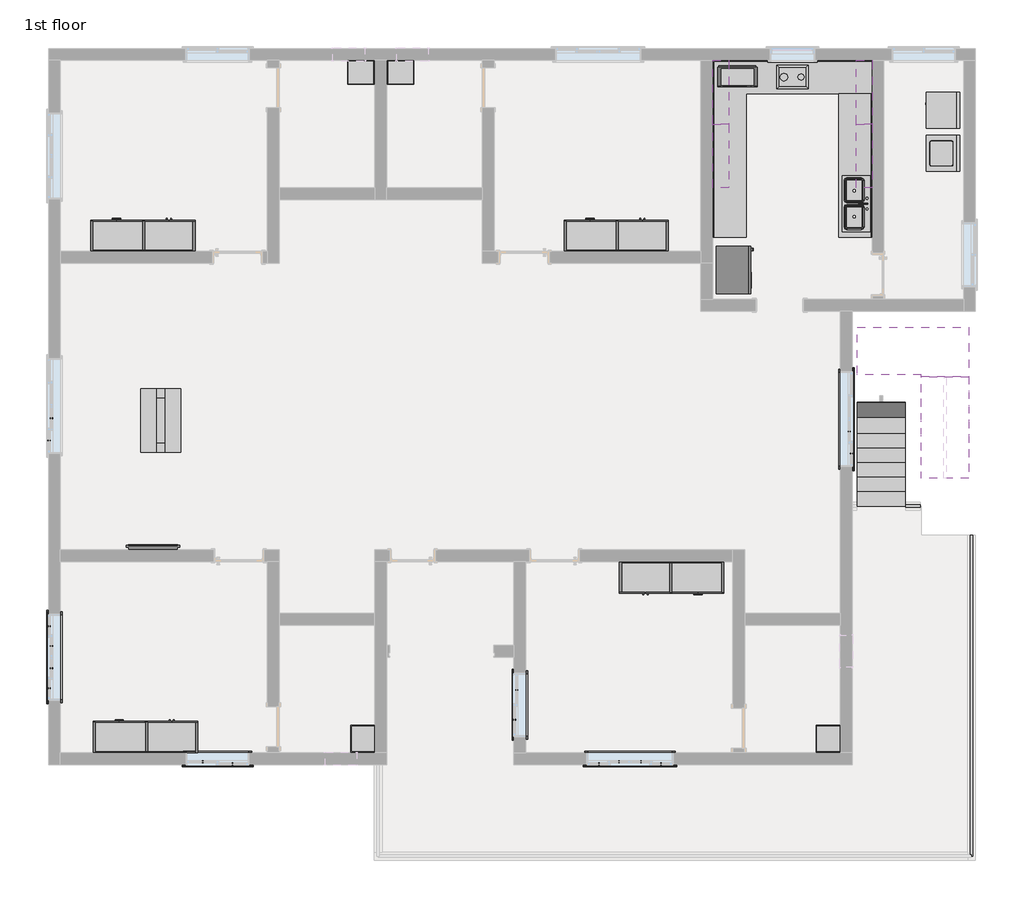
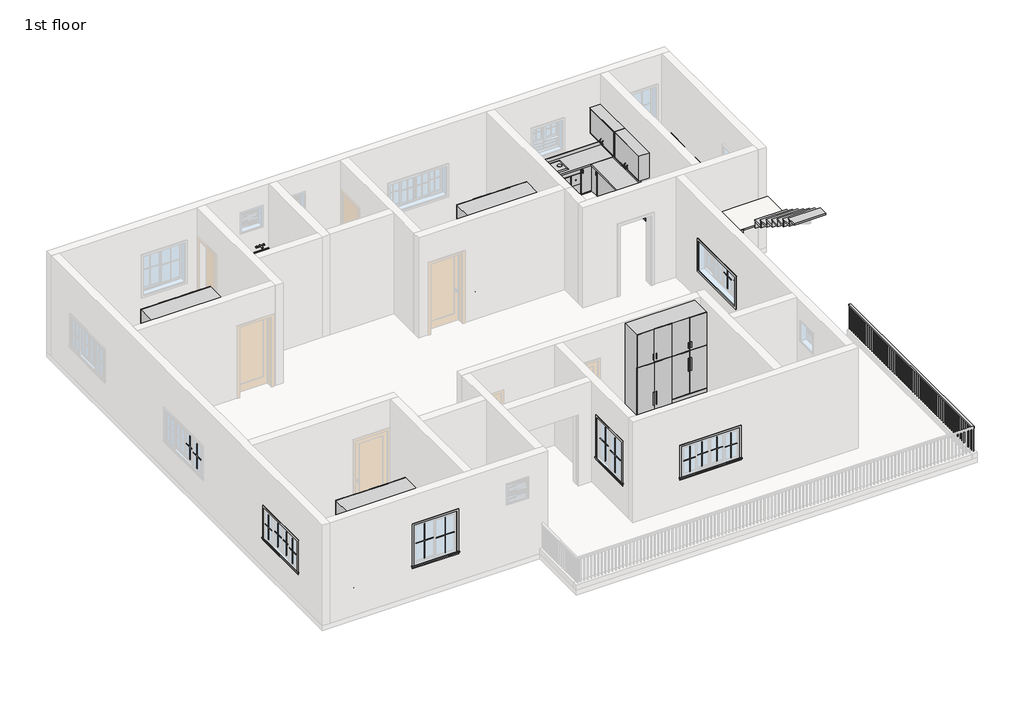
# One storey, part 3 of 4: 30 proxies, 19 furniture elements, 5 flow terminals, 2 railings, 2 stair flights, 1 slab.
"""IFC4 building model written with IfcOpenShell, lengths in millimetres."""

from ifc_helpers import new_model, si_unit, frame, origin, place, context, project, spatial, polyline, outline, extrude, transform, mapped, element, save
from components import proxy_3c1fa1d0, proxy_97c73763, proxy_e661f726, muntin_pattern_2x2_muntin_pattern_2x2_6186d23a, muntin_pattern_2x2_muntin_pattern_2x2_31a16349, muntin_pattern_2x2_muntin_pattern_2x2_cf37b409, trim_window_exterior_flat_with_sill_c3f87112, trim_window_exterior_flat_with_sill_3c945769, trim_window_exterior_flat_with_sill_7cfdd449, trim_window_interior_flat_picture_frame_1c33fa8a, trim_window_interior_flat_picture_frame_0edfbaa2, trim_window_interior_flat_picture_frame_f1e0b15b, proxy_e75280ca, flow_terminal_cce4e9d2, flow_terminal_a53be723, furniture_65fa61b5, furniture_1wardrobe_6271_1wardrobe_6271_4dd35231, furniture_3428e43d, furniture_97fe820d, furniture_803bf5e8, furniture_2797bbf7, furniture_b6aab1a0, furniture_ea954fa4, white_modern_coffee_table_17067_white_modern_coffee_table_d4aed9ff, non_monolithic_landing_cef278ae, stair_flight_508a9823, stair_flight_95b2deb1

model = new_model("IFC4")

# Units and contexts
model_context = context("Model", 3, world=origin())
ifc_project = project(units=[si_unit("LENGTHUNIT", "METRE", prefix="MILLI")], contexts=[model_context])

# Site, building, storey
site = spatial("IfcSite", under=ifc_project)
building = spatial("IfcBuilding", under=site)
storey = spatial("IfcBuildingStorey", under=building, Name="1st floor", Elevation=3810.0)

# Proxies
placement = place(None, origin())
proxy_shape = proxy_3c1fa1d0(model_context)
element("IfcBuildingElementProxy", 1, Name="Cook Top-2 Unit : 12\" x 18\" 2", ObjectType="Cook Top-2 Unit : 12\" x 18\" 2", at=placement, inside=storey, context=model_context, shape_type="MappedRepresentation", body=[
    mapped(proxy_shape, transform((6250.0508793, 6451.6660813, 3810.0), x_axis=(0.0, 1.0, 0.0), y_axis=(-1.0, 0.0, 0.0), z_axis=(0.0, 0.0, 1.0))),
])
proxy_2_shape = proxy_97c73763(model_context)
element("IfcBuildingElementProxy", 2, Name="Dryer : 27\" x 25\" x 35\"", ObjectType="Dryer : 27\" x 25\" x 35\"", at=placement, inside=storey, context=model_context, shape_type="MappedRepresentation", body=[
    mapped(proxy_2_shape, transform((8788.3284624, 6271.8535376, 3810.0), x_axis=(0.0, -1.0, 0.0), y_axis=(1.0, 0.0, 0.0), z_axis=(0.0, 0.0, 1.0))),
])
proxy_3_shape = proxy_e661f726(model_context)
element("IfcBuildingElementProxy", 3, Name="Microwave : 30\" x 16\" x 18\"", ObjectType="Microwave : 30\" x 16\" x 18\"", at=placement, inside=storey, context=model_context, shape_type="MappedRepresentation", body=[
    mapped(proxy_3_shape, transform((4665.4332064, 6893.6465872, 3810.0), x_axis=(1.0, 0.0, 0.0), y_axis=(0.0, 1.0, 0.0), z_axis=(0.0, 0.0, 1.0))),
])
muntin_pattern_2x2_muntin_pattern_2x2_shape = muntin_pattern_2x2_muntin_pattern_2x2_6186d23a(model_context)
element("IfcBuildingElementProxy", 4, Name="Muntin Pattern_2x2 : Muntin Pattern_2x2", ObjectType="Muntin Pattern_2x2 : Muntin Pattern_2x2", at=placement, inside=storey, context=model_context, shape_type="MappedRepresentation", body=[
    mapped(muntin_pattern_2x2_muntin_pattern_2x2_shape, transform((3702.0510838, -6632.5089187, 4806.95), x_axis=(-1.0, 0.0, 0.0), y_axis=(0.0, -1.0, 0.0), z_axis=(0.0, 0.0, 1.0))),
])
element("IfcBuildingElementProxy", 5, Name="Muntin Pattern_2x2 : Muntin Pattern_2x2", ObjectType="Muntin Pattern_2x2 : Muntin Pattern_2x2", at=placement, inside=storey, context=model_context, shape_type="MappedRepresentation", body=[
    mapped(muntin_pattern_2x2_muntin_pattern_2x2_shape, transform((3321.0510838, -6588.0589187, 4806.95), x_axis=(-1.0, 0.0, 0.0), y_axis=(0.0, -1.0, 0.0), z_axis=(0.0, 0.0, 1.0))),
])
element("IfcBuildingElementProxy", 6, Name="Muntin Pattern_2x2 : Muntin Pattern_2x2", ObjectType="Muntin Pattern_2x2 : Muntin Pattern_2x2", at=placement, inside=storey, context=model_context, shape_type="MappedRepresentation", body=[
    mapped(muntin_pattern_2x2_muntin_pattern_2x2_shape, transform((2895.6010838, -6588.0589187, 4806.95), x_axis=(-1.0, 0.0, 0.0), y_axis=(0.0, -1.0, 0.0), z_axis=(0.0, 0.0, 1.0))),
])
element("IfcBuildingElementProxy", 7, Name="Muntin Pattern_2x2 : Muntin Pattern_2x2", ObjectType="Muntin Pattern_2x2 : Muntin Pattern_2x2", at=placement, inside=storey, context=model_context, shape_type="MappedRepresentation", body=[
    mapped(muntin_pattern_2x2_muntin_pattern_2x2_shape, transform((2514.6010838, -6632.5089187, 4806.95), x_axis=(-1.0, 0.0, 0.0), y_axis=(0.0, -1.0, 0.0), z_axis=(0.0, 0.0, 1.0))),
])
element("IfcBuildingElementProxy", 8, Name="Muntin Pattern_2x2 : Muntin Pattern_2x2", ObjectType="Muntin Pattern_2x2 : Muntin Pattern_2x2", at=placement, inside=storey, context=model_context, shape_type="MappedRepresentation", body=[
    mapped(muntin_pattern_2x2_muntin_pattern_2x2_shape, transform((-8020.0489162, -5178.3589187, 4806.95), x_axis=(0.0, 1.0, 0.0), y_axis=(-1.0, 0.0, 0.0), z_axis=(0.0, 0.0, 1.0))),
])
element("IfcBuildingElementProxy", 9, Name="Muntin Pattern_2x2 : Muntin Pattern_2x2", ObjectType="Muntin Pattern_2x2 : Muntin Pattern_2x2", at=placement, inside=storey, context=model_context, shape_type="MappedRepresentation", body=[
    mapped(muntin_pattern_2x2_muntin_pattern_2x2_shape, transform((-7975.5989162, -4797.3589187, 4806.95), x_axis=(0.0, 1.0, 0.0), y_axis=(-1.0, 0.0, 0.0), z_axis=(0.0, 0.0, 1.0))),
])
element("IfcBuildingElementProxy", 10, Name="Muntin Pattern_2x2 : Muntin Pattern_2x2", ObjectType="Muntin Pattern_2x2 : Muntin Pattern_2x2", at=placement, inside=storey, context=model_context, shape_type="MappedRepresentation", body=[
    mapped(muntin_pattern_2x2_muntin_pattern_2x2_shape, transform((-7975.5989162, -4371.9089187, 4806.95), x_axis=(0.0, 1.0, 0.0), y_axis=(-1.0, 0.0, 0.0), z_axis=(0.0, 0.0, 1.0))),
])
element("IfcBuildingElementProxy", 11, Name="Muntin Pattern_2x2 : Muntin Pattern_2x2", ObjectType="Muntin Pattern_2x2 : Muntin Pattern_2x2", at=placement, inside=storey, context=model_context, shape_type="MappedRepresentation", body=[
    mapped(muntin_pattern_2x2_muntin_pattern_2x2_shape, transform((-8020.0489162, -3990.9089187, 4806.95), x_axis=(0.0, 1.0, 0.0), y_axis=(-1.0, 0.0, 0.0), z_axis=(0.0, 0.0, 1.0))),
])
muntin_pattern_2x2_muntin_pattern_2x2_2_shape = muntin_pattern_2x2_muntin_pattern_2x2_31a16349(model_context)
element("IfcBuildingElementProxy", 12, Name="Muntin Pattern_2x2 : Muntin Pattern_2x2", ObjectType="Muntin Pattern_2x2 : Muntin Pattern_2x2", at=placement, inside=storey, context=model_context, shape_type="MappedRepresentation", body=[
    mapped(muntin_pattern_2x2_muntin_pattern_2x2_2_shape, transform((-8020.0489162, -431.7339187, 4806.95), x_axis=(0.0, 1.0, 0.0), y_axis=(-1.0, 0.0, 0.0), z_axis=(0.0, 0.0, 1.0))),
])
element("IfcBuildingElementProxy", 13, Name="Muntin Pattern_2x2 : Muntin Pattern_2x2", ObjectType="Muntin Pattern_2x2 : Muntin Pattern_2x2", at=placement, inside=storey, context=model_context, shape_type="MappedRepresentation", body=[
    mapped(muntin_pattern_2x2_muntin_pattern_2x2_2_shape, transform((-7975.5989162, -6.2839187, 4806.95), x_axis=(0.0, 1.0, 0.0), y_axis=(-1.0, 0.0, 0.0), z_axis=(0.0, 0.0, 1.0))),
])
element("IfcBuildingElementProxy", 14, Name="Muntin Pattern_2x2 : Muntin Pattern_2x2", ObjectType="Muntin Pattern_2x2 : Muntin Pattern_2x2", at=placement, inside=storey, context=model_context, shape_type="MappedRepresentation", body=[
    mapped(muntin_pattern_2x2_muntin_pattern_2x2_2_shape, transform((7308.8510838, -260.2839187, 4806.95), x_axis=(0.0, -1.0, 0.0), y_axis=(1.0, 0.0, 0.0), z_axis=(0.0, 0.0, 1.0))),
])
element("IfcBuildingElementProxy", 15, Name="Muntin Pattern_2x2 : Muntin Pattern_2x2", ObjectType="Muntin Pattern_2x2 : Muntin Pattern_2x2", at=placement, inside=storey, context=model_context, shape_type="MappedRepresentation", body=[
    mapped(muntin_pattern_2x2_muntin_pattern_2x2_2_shape, transform((7353.3010838, -685.7339187, 4806.95), x_axis=(0.0, -1.0, 0.0), y_axis=(1.0, 0.0, 0.0), z_axis=(0.0, 0.0, 1.0))),
])
muntin_pattern_2x2_muntin_pattern_2x2_3_shape = muntin_pattern_2x2_muntin_pattern_2x2_cf37b409(model_context)
element("IfcBuildingElementProxy", 16, Name="Muntin Pattern_2x2 : Muntin Pattern_2x2", ObjectType="Muntin Pattern_2x2 : Muntin Pattern_2x2", at=placement, inside=storey, context=model_context, shape_type="MappedRepresentation", body=[
    mapped(muntin_pattern_2x2_muntin_pattern_2x2_3_shape, transform((939.8010838, -5214.8714187, 4806.95), x_axis=(0.0, 1.0, 0.0), y_axis=(-1.0, 0.0, 0.0), z_axis=(0.0, 0.0, 1.0))),
])
element("IfcBuildingElementProxy", 17, Name="Muntin Pattern_2x2 : Muntin Pattern_2x2", ObjectType="Muntin Pattern_2x2 : Muntin Pattern_2x2", at=placement, inside=storey, context=model_context, shape_type="MappedRepresentation", body=[
    mapped(muntin_pattern_2x2_muntin_pattern_2x2_3_shape, transform((895.3510838, -5783.1964187, 4806.95), x_axis=(0.0, 1.0, 0.0), y_axis=(-1.0, 0.0, 0.0), z_axis=(0.0, 0.0, 1.0))),
])
element("IfcBuildingElementProxy", 18, Name="Muntin Pattern_2x2 : Muntin Pattern_2x2", ObjectType="Muntin Pattern_2x2 : Muntin Pattern_2x2", at=placement, inside=storey, context=model_context, shape_type="MappedRepresentation", body=[
    mapped(muntin_pattern_2x2_muntin_pattern_2x2_3_shape, transform((-5075.2364162, -6588.0589187, 4806.95), x_axis=(-1.0, 0.0, 0.0), y_axis=(0.0, -1.0, 0.0), z_axis=(0.0, 0.0, 1.0))),
])
element("IfcBuildingElementProxy", 19, Name="Muntin Pattern_2x2 : Muntin Pattern_2x2", ObjectType="Muntin Pattern_2x2 : Muntin Pattern_2x2", at=placement, inside=storey, context=model_context, shape_type="MappedRepresentation", body=[
    mapped(muntin_pattern_2x2_muntin_pattern_2x2_3_shape, transform((-4506.9114162, -6632.5089187, 4806.95), x_axis=(-1.0, 0.0, 0.0), y_axis=(0.0, -1.0, 0.0), z_axis=(0.0, 0.0, 1.0))),
])
trim_window_exterior_flat_with_sill_shape = trim_window_exterior_flat_with_sill_c3f87112(model_context)
element("IfcBuildingElementProxy", 20, Name="Trim-Window-Exterior-Flat : with Sill", ObjectType="Trim-Window-Exterior-Flat : with Sill", at=placement, inside=storey, context=model_context, shape_type="MappedRepresentation", body=[
    mapped(trim_window_exterior_flat_with_sill_shape, transform((3108.3260838, -6642.0339187, 5638.8), x_axis=(1.0, 0.0, 0.0), y_axis=(0.0, 0.0, 1.0), z_axis=(0.0, -1.0, 0.0))),
])
element("IfcBuildingElementProxy", 21, Name="Trim-Window-Exterior-Flat : with Sill", ObjectType="Trim-Window-Exterior-Flat : with Sill", at=placement, inside=storey, context=model_context, shape_type="MappedRepresentation", body=[
    mapped(trim_window_exterior_flat_with_sill_shape, transform((-8029.5739162, -4584.6339187, 5638.8), x_axis=(0.0, -1.0, 0.0), y_axis=(0.0, 0.0, 1.0), z_axis=(-1.0, 0.0, 0.0))),
])
trim_window_exterior_flat_with_sill_2_shape = trim_window_exterior_flat_with_sill_3c945769(model_context)
element("IfcBuildingElementProxy", 22, Name="Trim-Window-Exterior-Flat : with Sill", ObjectType="Trim-Window-Exterior-Flat : with Sill", at=placement, inside=storey, context=model_context, shape_type="MappedRepresentation", body=[
    mapped(trim_window_exterior_flat_with_sill_2_shape, transform((7362.8260838, -25.3339187, 5638.8), x_axis=(0.0, 1.0, 0.0), y_axis=(0.0, 0.0, 1.0), z_axis=(1.0, 0.0, 0.0))),
])
trim_window_exterior_flat_with_sill_3_shape = trim_window_exterior_flat_with_sill_7cfdd449(model_context)
element("IfcBuildingElementProxy", 23, Name="Trim-Window-Exterior-Flat : with Sill", ObjectType="Trim-Window-Exterior-Flat : with Sill", at=placement, inside=storey, context=model_context, shape_type="MappedRepresentation", body=[
    mapped(trim_window_exterior_flat_with_sill_3_shape, transform((885.8260838, -5499.0339187, 5943.6), x_axis=(0.0, -1.0, 0.0), y_axis=(0.0, 0.0, 1.0), z_axis=(-1.0, 0.0, 0.0))),
])
element("IfcBuildingElementProxy", 24, Name="Trim-Window-Exterior-Flat : with Sill", ObjectType="Trim-Window-Exterior-Flat : with Sill", at=placement, inside=storey, context=model_context, shape_type="MappedRepresentation", body=[
    mapped(trim_window_exterior_flat_with_sill_3_shape, transform((-4791.0739162, -6642.0339187, 5943.6), x_axis=(1.0, 0.0, 0.0), y_axis=(0.0, 0.0, 1.0), z_axis=(0.0, -1.0, 0.0))),
])
trim_window_interior_flat_picture_frame_shape = trim_window_interior_flat_picture_frame_1c33fa8a(model_context)
element("IfcBuildingElementProxy", 25, Name="Trim-Window-Interior-Flat : Picture Frame", ObjectType="Trim-Window-Interior-Flat : Picture Frame", at=placement, inside=storey, context=model_context, shape_type="MappedRepresentation", body=[
    mapped(trim_window_interior_flat_picture_frame_shape, transform((3108.3260838, -6413.4339187, 5638.8), x_axis=(-1.0, 0.0, 0.0), y_axis=(0.0, 0.0, 1.0), z_axis=(0.0, 1.0, 0.0))),
])
element("IfcBuildingElementProxy", 26, Name="Trim-Window-Interior-Flat : Picture Frame", ObjectType="Trim-Window-Interior-Flat : Picture Frame", at=placement, inside=storey, context=model_context, shape_type="MappedRepresentation", body=[
    mapped(trim_window_interior_flat_picture_frame_shape, transform((-7800.9739162, -4584.6339187, 5638.8), x_axis=(0.0, 1.0, 0.0), y_axis=(0.0, 0.0, 1.0), z_axis=(1.0, 0.0, 0.0))),
])
trim_window_interior_flat_picture_frame_2_shape = trim_window_interior_flat_picture_frame_0edfbaa2(model_context)
element("IfcBuildingElementProxy", 27, Name="Trim-Window-Interior-Flat : Picture Frame", ObjectType="Trim-Window-Interior-Flat : Picture Frame", at=placement, inside=storey, context=model_context, shape_type="MappedRepresentation", body=[
    mapped(trim_window_interior_flat_picture_frame_2_shape, transform((7134.2260838, -25.3339187, 5638.8), x_axis=(0.0, -1.0, 0.0), y_axis=(0.0, 0.0, 1.0), z_axis=(-1.0, 0.0, 0.0))),
])
trim_window_interior_flat_picture_frame_3_shape = trim_window_interior_flat_picture_frame_f1e0b15b(model_context)
element("IfcBuildingElementProxy", 28, Name="Trim-Window-Interior-Flat : Picture Frame", ObjectType="Trim-Window-Interior-Flat : Picture Frame", at=placement, inside=storey, context=model_context, shape_type="MappedRepresentation", body=[
    mapped(trim_window_interior_flat_picture_frame_3_shape, transform((1114.4260838, -5499.0339187, 5943.6), x_axis=(0.0, 1.0, 0.0), y_axis=(0.0, 0.0, 1.0), z_axis=(1.0, 0.0, 0.0))),
])
element("IfcBuildingElementProxy", 29, Name="Trim-Window-Interior-Flat : Picture Frame", ObjectType="Trim-Window-Interior-Flat : Picture Frame", at=placement, inside=storey, context=model_context, shape_type="MappedRepresentation", body=[
    mapped(trim_window_interior_flat_picture_frame_3_shape, transform((-4791.0739162, -6413.4339187, 5943.6), x_axis=(-1.0, 0.0, 0.0), y_axis=(0.0, 0.0, 1.0), z_axis=(0.0, 1.0, 0.0))),
])
proxy_4_shape = proxy_e75280ca(model_context)
element("IfcBuildingElementProxy", 30, Name="Washer : 27\" x 25\" x 35\"", ObjectType="Washer : 27\" x 25\" x 35\"", at=placement, inside=storey, context=model_context, shape_type="MappedRepresentation", body=[
    mapped(proxy_4_shape, transform((8824.6435523, 5486.2156461, 3810.0), x_axis=(0.0, -1.0, 0.0), y_axis=(1.0, 0.0, 0.0), z_axis=(0.0, 0.0, 1.0))),
])

# Flow terminals
flow_terminal_shape = flow_terminal_cce4e9d2(model_context)
element("IfcFlowTerminal", 31, ObjectType="Sink - Work : 20\"x18\"", at=placement, inside=storey, context=model_context, shape_type="MappedRepresentation", body=[
    mapped(flow_terminal_shape, transform((-1285.8739162, 6845.3660813, 4724.4), x_axis=(1.0, 0.0, 0.0), y_axis=(0.0, 1.0, 0.0), z_axis=(0.0, 0.0, 1.0))),
])
element("IfcFlowTerminal", 32, ObjectType="Sink - Work : 20\"x18\"", at=placement, inside=storey, context=model_context, shape_type="MappedRepresentation", body=[
    mapped(flow_terminal_shape, transform((-2047.8739162, 6845.3660813, 4724.4), x_axis=(1.0, 0.0, 0.0), y_axis=(0.0, 1.0, 0.0), z_axis=(0.0, 0.0, 1.0))),
])
element("IfcFlowTerminal", 33, ObjectType="Sink - Work : 20\"x18\"", at=placement, inside=storey, context=model_context, shape_type="MappedRepresentation", body=[
    mapped(flow_terminal_shape, transform((-1781.1739162, -6146.7339187, 4724.4), x_axis=(0.0, -1.0, 0.0), y_axis=(1.0, 0.0, 0.0), z_axis=(0.0, 0.0, 1.0))),
])
element("IfcFlowTerminal", 34, ObjectType="Sink - Work : 20\"x18\"", at=placement, inside=storey, context=model_context, shape_type="MappedRepresentation", body=[
    mapped(flow_terminal_shape, transform((7134.2260838, -6146.7339187, 4724.4), x_axis=(0.0, -1.0, 0.0), y_axis=(1.0, 0.0, 0.0), z_axis=(0.0, 0.0, 1.0))),
])
flow_terminal_2_shape = flow_terminal_a53be723(model_context)
element("IfcFlowTerminal", 35, ObjectType="Sink Kitchen-Double : 42\" x 21\"", at=placement, inside=storey, context=model_context, shape_type="MappedRepresentation", body=[
    mapped(flow_terminal_2_shape, transform((7436.6806826, 4117.8553219, 3810.0), x_axis=(0.0, -1.0, 0.0), y_axis=(1.0, 0.0, 0.0), z_axis=(0.0, 0.0, 1.0))),
])

# Furniture
furniture_shape = furniture_65fa61b5(model_context)
element("IfcFurniture", 36, at=placement, inside=storey, context=model_context, shape_type="MappedRepresentation", body=[
    mapped(furniture_shape, transform((4759.3260838, 3441.7660813, 3810.0), x_axis=(0.0, 1.0, 0.0), y_axis=(-1.0, 0.0, 0.0), z_axis=(0.0, 0.0, 1.0))),
])
furniture_1wardrobe_6271_1wardrobe_6271_shape = furniture_1wardrobe_6271_1wardrobe_6271_4dd35231(model_context)
element("IfcFurniture", 37, ObjectType="1Wardrobe_6271 : 1Wardrobe_6271", at=placement, inside=storey, context=model_context, shape_type="MappedRepresentation", body=[
    mapped(furniture_1wardrobe_6271_1wardrobe_6271_shape, transform((-5222.8739162, 3187.7660813, 3810.0), x_axis=(-1.0, 0.0, 0.0), y_axis=(0.0, -1.0, 0.0), z_axis=(0.0, 0.0, 1.0))),
])
element("IfcFurniture", 38, ObjectType="1Wardrobe_6271 : 1Wardrobe_6271", at=placement, inside=storey, context=model_context, shape_type="MappedRepresentation", body=[
    mapped(furniture_1wardrobe_6271_1wardrobe_6271_shape, transform((3844.9260838, 3187.7660813, 3810.0), x_axis=(-1.0, 0.0, 0.0), y_axis=(0.0, -1.0, 0.0), z_axis=(0.0, 0.0, 1.0))),
])
element("IfcFurniture", 39, ObjectType="1Wardrobe_6271 : 1Wardrobe_6271", at=placement, inside=storey, context=model_context, shape_type="MappedRepresentation", body=[
    mapped(furniture_1wardrobe_6271_1wardrobe_6271_shape, transform((2905.1260838, -2755.8339187, 3810.0), x_axis=(1.0, 0.0, 0.0), y_axis=(0.0, 1.0, 0.0), z_axis=(0.0, 0.0, 1.0))),
])
element("IfcFurniture", 40, ObjectType="1Wardrobe_6271 : 1Wardrobe_6271", at=placement, inside=storey, context=model_context, shape_type="MappedRepresentation", body=[
    mapped(furniture_1wardrobe_6271_1wardrobe_6271_shape, transform((-5172.0739162, -6413.4339187, 3810.0), x_axis=(-1.0, 0.0, 0.0), y_axis=(0.0, -1.0, 0.0), z_axis=(0.0, 0.0, 1.0))),
])
furniture_2_shape = furniture_3428e43d(model_context)
element("IfcFurniture", 41, ObjectType="48\" 2", at=placement, inside=storey, context=model_context, shape_type="MappedRepresentation", body=[
    mapped(furniture_2_shape, transform((6128.9811238, 6845.3660813, 3810.0), x_axis=(1.0, 0.0, 0.0), y_axis=(0.0, 1.0, 0.0), z_axis=(0.0, 0.0, 1.0))),
])
element("IfcFurniture", 42, ObjectType="48\" 2", at=placement, inside=storey, context=model_context, shape_type="MappedRepresentation", body=[
    mapped(furniture_2_shape, transform((7134.2260838, 5230.5211213, 3810.0), x_axis=(0.0, 1.0, 0.0), y_axis=(-1.0, 0.0, 0.0), z_axis=(0.0, 0.0, 1.0))),
])
element("IfcFurniture", 43, ObjectType="48\" 2", at=placement, inside=storey, context=model_context, shape_type="MappedRepresentation", body=[
    mapped(furniture_2_shape, transform((4695.8260838, 5230.5211213, 3810.0), x_axis=(0.0, 1.0, 0.0), y_axis=(-1.0, 0.0, 0.0), z_axis=(0.0, 0.0, 1.0))),
])
element("IfcFurniture", 44, ObjectType="48\" 2", at=placement, inside=storey, context=model_context, shape_type="MappedRepresentation", body=[
    mapped(furniture_2_shape, transform((4695.8260838, 4011.3211213, 3810.0), x_axis=(0.0, 1.0, 0.0), y_axis=(-1.0, 0.0, 0.0), z_axis=(0.0, 0.0, 1.0))),
])
furniture_3_shape = furniture_97fe820d(model_context)
element("IfcFurniture", 45, ObjectType="Base Cabinet-Corner Unit-Square : 36\"", at=placement, inside=storey, context=model_context, shape_type="MappedRepresentation", body=[
    mapped(furniture_3_shape, transform((7217.0883788, 6845.3660813, 3810.0), x_axis=(1.0, 0.0, 0.0), y_axis=(0.0, 1.0, 0.0), z_axis=(0.0, 0.0, 1.0))),
])
element("IfcFurniture", 46, ObjectType="Base Cabinet-Corner Unit-Square : 36\"", at=placement, inside=storey, context=model_context, shape_type="MappedRepresentation", body=[
    mapped(furniture_3_shape, transform((4695.8260838, 6318.6283764, 3810.0), x_axis=(0.0, 1.0, 0.0), y_axis=(-1.0, 0.0, 0.0), z_axis=(0.0, 0.0, 1.0))),
])
furniture_4_shape = furniture_803bf5e8(model_context)
element("IfcFurniture", 47, ObjectType="Counter Top w Sink : 24\" Depth", at=placement, inside=storey, context=model_context, shape_type="MappedRepresentation", body=[
    mapped(furniture_4_shape, transform((7743.8260838, 5009.9037862, 3810.0), x_axis=(0.0, -1.0, 0.0), y_axis=(1.0, 0.0, 0.0), z_axis=(0.0, 0.0, 1.0))),
])
furniture_5_shape = furniture_2797bbf7(model_context)
element("IfcFurniture", 48, ObjectType="Counter Top-L Shaped : 24\" Depth", at=placement, inside=storey, context=model_context, shape_type="MappedRepresentation", body=[
    mapped(furniture_5_shape, transform((5896.2883788, 6845.3660813, 3810.0), x_axis=(1.0, 0.0, 0.0), y_axis=(0.0, 1.0, 0.0), z_axis=(0.0, 0.0, 1.0))),
])
furniture_6_shape = furniture_b6aab1a0(model_context)
element("IfcFurniture", 49, ObjectType="Television-Plasma : 42\"", at=placement, inside=storey, context=model_context, shape_type="MappedRepresentation", body=[
    mapped(furniture_6_shape, transform((-5972.1739162, -2527.2339187, 4876.8), x_axis=(-1.0, 0.0, 0.0), y_axis=(0.0, -1.0, 0.0), z_axis=(0.0, 0.0, 1.0))),
])
furniture_7_shape = furniture_ea954fa4(model_context)
element("IfcFurniture", 50, ObjectType="Upper Cabinet-Pass-Thru : 48\" x 30\" x 12\"", at=placement, inside=storey, context=model_context, shape_type="MappedRepresentation", body=[
    mapped(furniture_7_shape, transform((4695.8260838, 6217.0283764, 3810.0), x_axis=(0.0, 1.0, 0.0), y_axis=(-1.0, 0.0, 0.0), z_axis=(0.0, 0.0, 1.0))),
])
element("IfcFurniture", 51, ObjectType="Upper Cabinet-Pass-Thru : 48\" x 30\" x 12\"", at=placement, inside=storey, context=model_context, shape_type="MappedRepresentation", body=[
    mapped(furniture_7_shape, transform((4695.8260838, 4997.8283764, 3810.0), x_axis=(0.0, 1.0, 0.0), y_axis=(-1.0, 0.0, 0.0), z_axis=(0.0, 0.0, 1.0))),
])
element("IfcFurniture", 52, ObjectType="Upper Cabinet-Pass-Thru : 48\" x 30\" x 12\"", at=placement, inside=storey, context=model_context, shape_type="MappedRepresentation", body=[
    mapped(furniture_7_shape, transform((7743.8260838, 6254.5037862, 3810.0), x_axis=(0.0, -1.0, 0.0), y_axis=(1.0, 0.0, 0.0), z_axis=(0.0, 0.0, 1.0))),
])
element("IfcFurniture", 53, ObjectType="Upper Cabinet-Pass-Thru : 48\" x 30\" x 12\"", at=placement, inside=storey, context=model_context, shape_type="MappedRepresentation", body=[
    mapped(furniture_7_shape, transform((7743.8260838, 5035.3037862, 3810.0), x_axis=(0.0, -1.0, 0.0), y_axis=(1.0, 0.0, 0.0), z_axis=(0.0, 0.0, 1.0))),
])
white_modern_coffee_table_17067_white_modern_coffee_table_shape = white_modern_coffee_table_17067_white_modern_coffee_table_d4aed9ff(model_context)
element("IfcFurniture", 54, ObjectType="White_Modern_Coffee_Table_17067 : White_Modern_Coffee_Table_17067", at=placement, inside=storey, context=model_context, shape_type="MappedRepresentation", body=[
    mapped(white_modern_coffee_table_17067_white_modern_coffee_table_shape, transform((-5878.4127262, -50.7339187, 3810.0), x_axis=(0.0, 1.0, 0.0), y_axis=(-1.0, 0.0, 0.0), z_axis=(0.0, 0.0, 1.0))),
])

# Railings
element("IfcRailing", 55, ObjectType="Handrail - Rectangular", at=placement, inside=storey, context=model_context, shape_type="SweptSolid", body=[
    extrude(outline(polyline([(9623.4260838, -2247.8339187), (9674.2260838, -2247.8339187), (9674.2260838, -8394.6339187), (9623.4260838, -8394.6339187), (9623.4260838, -2247.8339187)])), frame((0.0, 0.0, 4673.6), z_axis=(0.0, 0.0, 1.0), x_axis=(1.0, 0.0, 0.0)), (0.0, 0.0, 1.0), 50.8),
    extrude(outline(polyline([(9639.3010838, -8334.3089187), (9658.3510838, -8334.3089187), (9658.3510838, -8353.3589187), (9639.3010838, -8353.3589187), (9639.3010838, -8334.3089187)])), frame((0.0, 0.0, 3810.0), z_axis=(0.0, 0.0, 1.0), x_axis=(1.0, 0.0, 0.0)), (0.0, 0.0, 1.0), 863.6),
    extrude(outline(polyline([(9639.3010838, -8232.7089187), (9658.3510838, -8232.7089187), (9658.3510838, -8251.7589187), (9639.3010838, -8251.7589187), (9639.3010838, -8232.7089187)])), frame((0.0, 0.0, 3810.0), z_axis=(0.0, 0.0, 1.0), x_axis=(1.0, 0.0, 0.0)), (0.0, 0.0, 1.0), 863.6),
    extrude(outline(polyline([(9639.3010838, -8131.1089187), (9658.3510838, -8131.1089187), (9658.3510838, -8150.1589187), (9639.3010838, -8150.1589187), (9639.3010838, -8131.1089187)])), frame((0.0, 0.0, 3810.0), z_axis=(0.0, 0.0, 1.0), x_axis=(1.0, 0.0, 0.0)), (0.0, 0.0, 1.0), 863.6),
    extrude(outline(polyline([(9639.3010838, -8029.5089187), (9658.3510838, -8029.5089187), (9658.3510838, -8048.5589187), (9639.3010838, -8048.5589187), (9639.3010838, -8029.5089187)])), frame((0.0, 0.0, 3810.0), z_axis=(0.0, 0.0, 1.0), x_axis=(1.0, 0.0, 0.0)), (0.0, 0.0, 1.0), 863.6),
    extrude(outline(polyline([(9639.3010838, -7927.9089187), (9658.3510838, -7927.9089187), (9658.3510838, -7946.9589187), (9639.3010838, -7946.9589187), (9639.3010838, -7927.9089187)])), frame((0.0, 0.0, 3810.0), z_axis=(0.0, 0.0, 1.0), x_axis=(1.0, 0.0, 0.0)), (0.0, 0.0, 1.0), 863.6),
    extrude(outline(polyline([(9639.3010838, -7826.3089187), (9658.3510838, -7826.3089187), (9658.3510838, -7845.3589187), (9639.3010838, -7845.3589187), (9639.3010838, -7826.3089187)])), frame((0.0, 0.0, 3810.0), z_axis=(0.0, 0.0, 1.0), x_axis=(1.0, 0.0, 0.0)), (0.0, 0.0, 1.0), 863.6),
    extrude(outline(polyline([(9639.3010838, -7724.7089187), (9658.3510838, -7724.7089187), (9658.3510838, -7743.7589187), (9639.3010838, -7743.7589187), (9639.3010838, -7724.7089187)])), frame((0.0, 0.0, 3810.0), z_axis=(0.0, 0.0, 1.0), x_axis=(1.0, 0.0, 0.0)), (0.0, 0.0, 1.0), 863.6),
    extrude(outline(polyline([(9639.3010838, -7623.1089187), (9658.3510838, -7623.1089187), (9658.3510838, -7642.1589187), (9639.3010838, -7642.1589187), (9639.3010838, -7623.1089187)])), frame((0.0, 0.0, 3810.0), z_axis=(0.0, 0.0, 1.0), x_axis=(1.0, 0.0, 0.0)), (0.0, 0.0, 1.0), 863.6),
    extrude(outline(polyline([(9639.3010838, -7521.5089187), (9658.3510838, -7521.5089187), (9658.3510838, -7540.5589187), (9639.3010838, -7540.5589187), (9639.3010838, -7521.5089187)])), frame((0.0, 0.0, 3810.0), z_axis=(0.0, 0.0, 1.0), x_axis=(1.0, 0.0, 0.0)), (0.0, 0.0, 1.0), 863.6),
    extrude(outline(polyline([(9639.3010838, -7419.9089187), (9658.3510838, -7419.9089187), (9658.3510838, -7438.9589187), (9639.3010838, -7438.9589187), (9639.3010838, -7419.9089187)])), frame((0.0, 0.0, 3810.0), z_axis=(0.0, 0.0, 1.0), x_axis=(1.0, 0.0, 0.0)), (0.0, 0.0, 1.0), 863.6),
    extrude(outline(polyline([(9639.3010838, -7318.3089187), (9658.3510838, -7318.3089187), (9658.3510838, -7337.3589187), (9639.3010838, -7337.3589187), (9639.3010838, -7318.3089187)])), frame((0.0, 0.0, 3810.0), z_axis=(0.0, 0.0, 1.0), x_axis=(1.0, 0.0, 0.0)), (0.0, 0.0, 1.0), 863.6),
    extrude(outline(polyline([(9639.3010838, -7216.7089187), (9658.3510838, -7216.7089187), (9658.3510838, -7235.7589187), (9639.3010838, -7235.7589187), (9639.3010838, -7216.7089187)])), frame((0.0, 0.0, 3810.0), z_axis=(0.0, 0.0, 1.0), x_axis=(1.0, 0.0, 0.0)), (0.0, 0.0, 1.0), 863.6),
    extrude(outline(polyline([(9639.3010838, -7115.1089187), (9658.3510838, -7115.1089187), (9658.3510838, -7134.1589187), (9639.3010838, -7134.1589187), (9639.3010838, -7115.1089187)])), frame((0.0, 0.0, 3810.0), z_axis=(0.0, 0.0, 1.0), x_axis=(1.0, 0.0, 0.0)), (0.0, 0.0, 1.0), 863.6),
    extrude(outline(polyline([(9639.3010838, -7013.5089187), (9658.3510838, -7013.5089187), (9658.3510838, -7032.5589187), (9639.3010838, -7032.5589187), (9639.3010838, -7013.5089187)])), frame((0.0, 0.0, 3810.0), z_axis=(0.0, 0.0, 1.0), x_axis=(1.0, 0.0, 0.0)), (0.0, 0.0, 1.0), 863.6),
    extrude(outline(polyline([(9639.3010838, -6911.9089187), (9658.3510838, -6911.9089187), (9658.3510838, -6930.9589187), (9639.3010838, -6930.9589187), (9639.3010838, -6911.9089187)])), frame((0.0, 0.0, 3810.0), z_axis=(0.0, 0.0, 1.0), x_axis=(1.0, 0.0, 0.0)), (0.0, 0.0, 1.0), 863.6),
    extrude(outline(polyline([(9639.3010838, -6810.3089187), (9658.3510838, -6810.3089187), (9658.3510838, -6829.3589187), (9639.3010838, -6829.3589187), (9639.3010838, -6810.3089187)])), frame((0.0, 0.0, 3810.0), z_axis=(0.0, 0.0, 1.0), x_axis=(1.0, 0.0, 0.0)), (0.0, 0.0, 1.0), 863.6),
    extrude(outline(polyline([(9639.3010838, -6708.7089187), (9658.3510838, -6708.7089187), (9658.3510838, -6727.7589187), (9639.3010838, -6727.7589187), (9639.3010838, -6708.7089187)])), frame((0.0, 0.0, 3810.0), z_axis=(0.0, 0.0, 1.0), x_axis=(1.0, 0.0, 0.0)), (0.0, 0.0, 1.0), 863.6),
    extrude(outline(polyline([(9639.3010838, -6607.1089187), (9658.3510838, -6607.1089187), (9658.3510838, -6626.1589187), (9639.3010838, -6626.1589187), (9639.3010838, -6607.1089187)])), frame((0.0, 0.0, 3810.0), z_axis=(0.0, 0.0, 1.0), x_axis=(1.0, 0.0, 0.0)), (0.0, 0.0, 1.0), 863.6),
    extrude(outline(polyline([(9639.3010838, -6505.5089187), (9658.3510838, -6505.5089187), (9658.3510838, -6524.5589187), (9639.3010838, -6524.5589187), (9639.3010838, -6505.5089187)])), frame((0.0, 0.0, 3810.0), z_axis=(0.0, 0.0, 1.0), x_axis=(1.0, 0.0, 0.0)), (0.0, 0.0, 1.0), 863.6),
    extrude(outline(polyline([(9639.3010838, -6403.9089187), (9658.3510838, -6403.9089187), (9658.3510838, -6422.9589187), (9639.3010838, -6422.9589187), (9639.3010838, -6403.9089187)])), frame((0.0, 0.0, 3810.0), z_axis=(0.0, 0.0, 1.0), x_axis=(1.0, 0.0, 0.0)), (0.0, 0.0, 1.0), 863.6),
    extrude(outline(polyline([(9639.3010838, -6302.3089187), (9658.3510838, -6302.3089187), (9658.3510838, -6321.3589187), (9639.3010838, -6321.3589187), (9639.3010838, -6302.3089187)])), frame((0.0, 0.0, 3810.0), z_axis=(0.0, 0.0, 1.0), x_axis=(1.0, 0.0, 0.0)), (0.0, 0.0, 1.0), 863.6),
    extrude(outline(polyline([(9639.3010838, -6200.7089187), (9658.3510838, -6200.7089187), (9658.3510838, -6219.7589187), (9639.3010838, -6219.7589187), (9639.3010838, -6200.7089187)])), frame((0.0, 0.0, 3810.0), z_axis=(0.0, 0.0, 1.0), x_axis=(1.0, 0.0, 0.0)), (0.0, 0.0, 1.0), 863.6),
    extrude(outline(polyline([(9639.3010838, -6099.1089187), (9658.3510838, -6099.1089187), (9658.3510838, -6118.1589187), (9639.3010838, -6118.1589187), (9639.3010838, -6099.1089187)])), frame((0.0, 0.0, 3810.0), z_axis=(0.0, 0.0, 1.0), x_axis=(1.0, 0.0, 0.0)), (0.0, 0.0, 1.0), 863.6),
    extrude(outline(polyline([(9639.3010838, -5997.5089187), (9658.3510838, -5997.5089187), (9658.3510838, -6016.5589187), (9639.3010838, -6016.5589187), (9639.3010838, -5997.5089187)])), frame((0.0, 0.0, 3810.0), z_axis=(0.0, 0.0, 1.0), x_axis=(1.0, 0.0, 0.0)), (0.0, 0.0, 1.0), 863.6),
    extrude(outline(polyline([(9639.3010838, -5895.9089187), (9658.3510838, -5895.9089187), (9658.3510838, -5914.9589187), (9639.3010838, -5914.9589187), (9639.3010838, -5895.9089187)])), frame((0.0, 0.0, 3810.0), z_axis=(0.0, 0.0, 1.0), x_axis=(1.0, 0.0, 0.0)), (0.0, 0.0, 1.0), 863.6),
    extrude(outline(polyline([(9639.3010838, -5794.3089187), (9658.3510838, -5794.3089187), (9658.3510838, -5813.3589187), (9639.3010838, -5813.3589187), (9639.3010838, -5794.3089187)])), frame((0.0, 0.0, 3810.0), z_axis=(0.0, 0.0, 1.0), x_axis=(1.0, 0.0, 0.0)), (0.0, 0.0, 1.0), 863.6),
    extrude(outline(polyline([(9639.3010838, -5692.7089187), (9658.3510838, -5692.7089187), (9658.3510838, -5711.7589187), (9639.3010838, -5711.7589187), (9639.3010838, -5692.7089187)])), frame((0.0, 0.0, 3810.0), z_axis=(0.0, 0.0, 1.0), x_axis=(1.0, 0.0, 0.0)), (0.0, 0.0, 1.0), 863.6),
    extrude(outline(polyline([(9639.3010838, -5591.1089187), (9658.3510838, -5591.1089187), (9658.3510838, -5610.1589187), (9639.3010838, -5610.1589187), (9639.3010838, -5591.1089187)])), frame((0.0, 0.0, 3810.0), z_axis=(0.0, 0.0, 1.0), x_axis=(1.0, 0.0, 0.0)), (0.0, 0.0, 1.0), 863.6),
    extrude(outline(polyline([(9639.3010838, -5489.5089187), (9658.3510838, -5489.5089187), (9658.3510838, -5508.5589187), (9639.3010838, -5508.5589187), (9639.3010838, -5489.5089187)])), frame((0.0, 0.0, 3810.0), z_axis=(0.0, 0.0, 1.0), x_axis=(1.0, 0.0, 0.0)), (0.0, 0.0, 1.0), 863.6),
    extrude(outline(polyline([(9639.3010838, -5387.9089187), (9658.3510838, -5387.9089187), (9658.3510838, -5406.9589187), (9639.3010838, -5406.9589187), (9639.3010838, -5387.9089187)])), frame((0.0, 0.0, 3810.0), z_axis=(0.0, 0.0, 1.0), x_axis=(1.0, 0.0, 0.0)), (0.0, 0.0, 1.0), 863.6),
    extrude(outline(polyline([(9639.3010838, -5286.3089187), (9658.3510838, -5286.3089187), (9658.3510838, -5305.3589187), (9639.3010838, -5305.3589187), (9639.3010838, -5286.3089187)])), frame((0.0, 0.0, 3810.0), z_axis=(0.0, 0.0, 1.0), x_axis=(1.0, 0.0, 0.0)), (0.0, 0.0, 1.0), 863.6),
    extrude(outline(polyline([(9639.3010838, -5184.7089187), (9658.3510838, -5184.7089187), (9658.3510838, -5203.7589187), (9639.3010838, -5203.7589187), (9639.3010838, -5184.7089187)])), frame((0.0, 0.0, 3810.0), z_axis=(0.0, 0.0, 1.0), x_axis=(1.0, 0.0, 0.0)), (0.0, 0.0, 1.0), 863.6),
    extrude(outline(polyline([(9639.3010838, -5083.1089187), (9658.3510838, -5083.1089187), (9658.3510838, -5102.1589187), (9639.3010838, -5102.1589187), (9639.3010838, -5083.1089187)])), frame((0.0, 0.0, 3810.0), z_axis=(0.0, 0.0, 1.0), x_axis=(1.0, 0.0, 0.0)), (0.0, 0.0, 1.0), 863.6),
    extrude(outline(polyline([(9639.3010838, -4981.5089187), (9658.3510838, -4981.5089187), (9658.3510838, -5000.5589187), (9639.3010838, -5000.5589187), (9639.3010838, -4981.5089187)])), frame((0.0, 0.0, 3810.0), z_axis=(0.0, 0.0, 1.0), x_axis=(1.0, 0.0, 0.0)), (0.0, 0.0, 1.0), 863.6),
    extrude(outline(polyline([(9639.3010838, -4879.9089187), (9658.3510838, -4879.9089187), (9658.3510838, -4898.9589187), (9639.3010838, -4898.9589187), (9639.3010838, -4879.9089187)])), frame((0.0, 0.0, 3810.0), z_axis=(0.0, 0.0, 1.0), x_axis=(1.0, 0.0, 0.0)), (0.0, 0.0, 1.0), 863.6),
    extrude(outline(polyline([(9639.3010838, -4778.3089187), (9658.3510838, -4778.3089187), (9658.3510838, -4797.3589187), (9639.3010838, -4797.3589187), (9639.3010838, -4778.3089187)])), frame((0.0, 0.0, 3810.0), z_axis=(0.0, 0.0, 1.0), x_axis=(1.0, 0.0, 0.0)), (0.0, 0.0, 1.0), 863.6),
    extrude(outline(polyline([(9639.3010838, -4676.7089187), (9658.3510838, -4676.7089187), (9658.3510838, -4695.7589187), (9639.3010838, -4695.7589187), (9639.3010838, -4676.7089187)])), frame((0.0, 0.0, 3810.0), z_axis=(0.0, 0.0, 1.0), x_axis=(1.0, 0.0, 0.0)), (0.0, 0.0, 1.0), 863.6),
    extrude(outline(polyline([(9639.3010838, -4575.1089187), (9658.3510838, -4575.1089187), (9658.3510838, -4594.1589187), (9639.3010838, -4594.1589187), (9639.3010838, -4575.1089187)])), frame((0.0, 0.0, 3810.0), z_axis=(0.0, 0.0, 1.0), x_axis=(1.0, 0.0, 0.0)), (0.0, 0.0, 1.0), 863.6),
    extrude(outline(polyline([(9639.3010838, -4473.5089187), (9658.3510838, -4473.5089187), (9658.3510838, -4492.5589187), (9639.3010838, -4492.5589187), (9639.3010838, -4473.5089187)])), frame((0.0, 0.0, 3810.0), z_axis=(0.0, 0.0, 1.0), x_axis=(1.0, 0.0, 0.0)), (0.0, 0.0, 1.0), 863.6),
    extrude(outline(polyline([(9639.3010838, -4371.9089187), (9658.3510838, -4371.9089187), (9658.3510838, -4390.9589187), (9639.3010838, -4390.9589187), (9639.3010838, -4371.9089187)])), frame((0.0, 0.0, 3810.0), z_axis=(0.0, 0.0, 1.0), x_axis=(1.0, 0.0, 0.0)), (0.0, 0.0, 1.0), 863.6),
    extrude(outline(polyline([(9639.3010838, -4270.3089187), (9658.3510838, -4270.3089187), (9658.3510838, -4289.3589187), (9639.3010838, -4289.3589187), (9639.3010838, -4270.3089187)])), frame((0.0, 0.0, 3810.0), z_axis=(0.0, 0.0, 1.0), x_axis=(1.0, 0.0, 0.0)), (0.0, 0.0, 1.0), 863.6),
    extrude(outline(polyline([(9639.3010838, -4168.7089187), (9658.3510838, -4168.7089187), (9658.3510838, -4187.7589187), (9639.3010838, -4187.7589187), (9639.3010838, -4168.7089187)])), frame((0.0, 0.0, 3810.0), z_axis=(0.0, 0.0, 1.0), x_axis=(1.0, 0.0, 0.0)), (0.0, 0.0, 1.0), 863.6),
    extrude(outline(polyline([(9639.3010838, -4067.1089187), (9658.3510838, -4067.1089187), (9658.3510838, -4086.1589187), (9639.3010838, -4086.1589187), (9639.3010838, -4067.1089187)])), frame((0.0, 0.0, 3810.0), z_axis=(0.0, 0.0, 1.0), x_axis=(1.0, 0.0, 0.0)), (0.0, 0.0, 1.0), 863.6),
    extrude(outline(polyline([(9639.3010838, -3965.5089187), (9658.3510838, -3965.5089187), (9658.3510838, -3984.5589187), (9639.3010838, -3984.5589187), (9639.3010838, -3965.5089187)])), frame((0.0, 0.0, 3810.0), z_axis=(0.0, 0.0, 1.0), x_axis=(1.0, 0.0, 0.0)), (0.0, 0.0, 1.0), 863.6),
    extrude(outline(polyline([(9639.3010838, -3863.9089187), (9658.3510838, -3863.9089187), (9658.3510838, -3882.9589187), (9639.3010838, -3882.9589187), (9639.3010838, -3863.9089187)])), frame((0.0, 0.0, 3810.0), z_axis=(0.0, 0.0, 1.0), x_axis=(1.0, 0.0, 0.0)), (0.0, 0.0, 1.0), 863.6),
    extrude(outline(polyline([(9639.3010838, -3762.3089187), (9658.3510838, -3762.3089187), (9658.3510838, -3781.3589187), (9639.3010838, -3781.3589187), (9639.3010838, -3762.3089187)])), frame((0.0, 0.0, 3810.0), z_axis=(0.0, 0.0, 1.0), x_axis=(1.0, 0.0, 0.0)), (0.0, 0.0, 1.0), 863.6),
    extrude(outline(polyline([(9639.3010838, -3660.7089187), (9658.3510838, -3660.7089187), (9658.3510838, -3679.7589187), (9639.3010838, -3679.7589187), (9639.3010838, -3660.7089187)])), frame((0.0, 0.0, 3810.0), z_axis=(0.0, 0.0, 1.0), x_axis=(1.0, 0.0, 0.0)), (0.0, 0.0, 1.0), 863.6),
    extrude(outline(polyline([(9639.3010838, -3559.1089187), (9658.3510838, -3559.1089187), (9658.3510838, -3578.1589187), (9639.3010838, -3578.1589187), (9639.3010838, -3559.1089187)])), frame((0.0, 0.0, 3810.0), z_axis=(0.0, 0.0, 1.0), x_axis=(1.0, 0.0, 0.0)), (0.0, 0.0, 1.0), 863.6),
    extrude(outline(polyline([(9639.3010838, -3457.5089187), (9658.3510838, -3457.5089187), (9658.3510838, -3476.5589187), (9639.3010838, -3476.5589187), (9639.3010838, -3457.5089187)])), frame((0.0, 0.0, 3810.0), z_axis=(0.0, 0.0, 1.0), x_axis=(1.0, 0.0, 0.0)), (0.0, 0.0, 1.0), 863.6),
    extrude(outline(polyline([(9639.3010838, -3355.9089187), (9658.3510838, -3355.9089187), (9658.3510838, -3374.9589187), (9639.3010838, -3374.9589187), (9639.3010838, -3355.9089187)])), frame((0.0, 0.0, 3810.0), z_axis=(0.0, 0.0, 1.0), x_axis=(1.0, 0.0, 0.0)), (0.0, 0.0, 1.0), 863.6),
    extrude(outline(polyline([(9639.3010838, -3254.3089187), (9658.3510838, -3254.3089187), (9658.3510838, -3273.3589187), (9639.3010838, -3273.3589187), (9639.3010838, -3254.3089187)])), frame((0.0, 0.0, 3810.0), z_axis=(0.0, 0.0, 1.0), x_axis=(1.0, 0.0, 0.0)), (0.0, 0.0, 1.0), 863.6),
    extrude(outline(polyline([(9639.3010838, -3152.7089187), (9658.3510838, -3152.7089187), (9658.3510838, -3171.7589187), (9639.3010838, -3171.7589187), (9639.3010838, -3152.7089187)])), frame((0.0, 0.0, 3810.0), z_axis=(0.0, 0.0, 1.0), x_axis=(1.0, 0.0, 0.0)), (0.0, 0.0, 1.0), 863.6),
    extrude(outline(polyline([(9639.3010838, -3051.1089187), (9658.3510838, -3051.1089187), (9658.3510838, -3070.1589187), (9639.3010838, -3070.1589187), (9639.3010838, -3051.1089187)])), frame((0.0, 0.0, 3810.0), z_axis=(0.0, 0.0, 1.0), x_axis=(1.0, 0.0, 0.0)), (0.0, 0.0, 1.0), 863.6),
    extrude(outline(polyline([(9639.3010838, -2949.5089187), (9658.3510838, -2949.5089187), (9658.3510838, -2968.5589187), (9639.3010838, -2968.5589187), (9639.3010838, -2949.5089187)])), frame((0.0, 0.0, 3810.0), z_axis=(0.0, 0.0, 1.0), x_axis=(1.0, 0.0, 0.0)), (0.0, 0.0, 1.0), 863.6),
    extrude(outline(polyline([(9639.3010838, -2847.9089187), (9658.3510838, -2847.9089187), (9658.3510838, -2866.9589187), (9639.3010838, -2866.9589187), (9639.3010838, -2847.9089187)])), frame((0.0, 0.0, 3810.0), z_axis=(0.0, 0.0, 1.0), x_axis=(1.0, 0.0, 0.0)), (0.0, 0.0, 1.0), 863.6),
    extrude(outline(polyline([(9639.3010838, -2746.3089187), (9658.3510838, -2746.3089187), (9658.3510838, -2765.3589187), (9639.3010838, -2765.3589187), (9639.3010838, -2746.3089187)])), frame((0.0, 0.0, 3810.0), z_axis=(0.0, 0.0, 1.0), x_axis=(1.0, 0.0, 0.0)), (0.0, 0.0, 1.0), 863.6),
    extrude(outline(polyline([(9639.3010838, -2644.7089187), (9658.3510838, -2644.7089187), (9658.3510838, -2663.7589187), (9639.3010838, -2663.7589187), (9639.3010838, -2644.7089187)])), frame((0.0, 0.0, 3810.0), z_axis=(0.0, 0.0, 1.0), x_axis=(1.0, 0.0, 0.0)), (0.0, 0.0, 1.0), 863.6),
    extrude(outline(polyline([(9639.3010838, -2543.1089187), (9658.3510838, -2543.1089187), (9658.3510838, -2562.1589187), (9639.3010838, -2562.1589187), (9639.3010838, -2543.1089187)])), frame((0.0, 0.0, 3810.0), z_axis=(0.0, 0.0, 1.0), x_axis=(1.0, 0.0, 0.0)), (0.0, 0.0, 1.0), 863.6),
    extrude(outline(polyline([(9639.3010838, -2441.5089187), (9658.3510838, -2441.5089187), (9658.3510838, -2460.5589187), (9639.3010838, -2460.5589187), (9639.3010838, -2441.5089187)])), frame((0.0, 0.0, 3810.0), z_axis=(0.0, 0.0, 1.0), x_axis=(1.0, 0.0, 0.0)), (0.0, 0.0, 1.0), 863.6),
    extrude(outline(polyline([(9639.3010838, -2339.9089187), (9658.3510838, -2339.9089187), (9658.3510838, -2358.9589187), (9639.3010838, -2358.9589187), (9639.3010838, -2339.9089187)])), frame((0.0, 0.0, 3810.0), z_axis=(0.0, 0.0, 1.0), x_axis=(1.0, 0.0, 0.0)), (0.0, 0.0, 1.0), 863.6),
    extrude(outline(polyline([(9639.3010838, -8375.5839187), (9658.3510838, -8375.5839187), (9658.3510838, -8394.6339187), (9639.3010838, -8394.6339187), (9639.3010838, -8375.5839187)])), frame((0.0, 0.0, 3810.0), z_axis=(0.0, 0.0, 1.0), x_axis=(1.0, 0.0, 0.0)), (0.0, 0.0, 1.0), 863.6),
    extrude(outline(polyline([(9639.3010838, -2247.8339187), (9658.3510838, -2247.8339187), (9658.3510838, -2266.8839187), (9639.3010838, -2266.8839187), (9639.3010838, -2247.8339187)])), frame((0.0, 0.0, 3810.0), z_axis=(0.0, 0.0, 1.0), x_axis=(1.0, 0.0, 0.0)), (0.0, 0.0, 1.0), 863.6),
])
element("IfcRailing", 56, ObjectType="Handrail - Rectangular", at=placement, inside=storey, context=model_context, shape_type="SweptSolid", body=[
    extrude(outline(polyline([(8391.5260838, -1714.4339187), (8391.5260838, -1663.6339187), (8670.9260838, -1663.6339187), (8670.9260838, -1714.4339187), (8391.5260838, -1714.4339187)])), frame((0.0, 0.0, 4673.6), z_axis=(0.0, 0.0, 1.0), x_axis=(1.0, 0.0, 0.0)), (0.0, 0.0, 1.0), 50.8),
    extrude(outline(polyline([(8585.2010838, -1698.5589187), (8585.2010838, -1679.5089187), (8604.2510838, -1679.5089187), (8604.2510838, -1698.5589187), (8585.2010838, -1698.5589187)])), frame((0.0, 0.0, 3810.0), z_axis=(0.0, 0.0, 1.0), x_axis=(1.0, 0.0, 0.0)), (0.0, 0.0, 1.0), 863.6),
    extrude(outline(polyline([(8483.6010838, -1698.5589187), (8483.6010838, -1679.5089187), (8502.6510838, -1679.5089187), (8502.6510838, -1698.5589187), (8483.6010838, -1698.5589187)])), frame((0.0, 0.0, 3810.0), z_axis=(0.0, 0.0, 1.0), x_axis=(1.0, 0.0, 0.0)), (0.0, 0.0, 1.0), 863.6),
    extrude(outline(polyline([(8651.8760838, -1698.5589187), (8651.8760838, -1679.5089187), (8670.9260838, -1679.5089187), (8670.9260838, -1698.5589187), (8651.8760838, -1698.5589187)])), frame((0.0, 0.0, 3810.0), z_axis=(0.0, 0.0, 1.0), x_axis=(1.0, 0.0, 0.0)), (0.0, 0.0, 1.0), 863.6),
    extrude(outline(polyline([(8391.5260838, -1698.5589187), (8391.5260838, -1679.5089187), (8410.5760838, -1679.5089187), (8410.5760838, -1698.5589187), (8391.5260838, -1698.5589187)])), frame((0.0, 0.0, 3810.0), z_axis=(0.0, 0.0, 1.0), x_axis=(1.0, 0.0, 0.0)), (0.0, 0.0, 1.0), 863.6),
])

# Slab
non_monolithic_landing_shape = non_monolithic_landing_cef278ae(model_context)
element("IfcSlab", 57, ObjectType="Non-Monolithic Landing", at=placement, inside=storey, context=model_context, shape_type="MappedRepresentation", body=[
    mapped(non_monolithic_landing_shape, transform((0.0, 0.0, 0.0), x_axis=(1.0, 0.0, 0.0), y_axis=(0.0, 1.0, 0.0), z_axis=(0.0, 0.0, 1.0))),
])

# Stair flights
stair_flight_shape = stair_flight_508a9823(model_context)
element("IfcStairFlight", 58, ObjectType="2\" Tread 1\" Nosing 1/4\" Riser", at=placement, inside=storey, context=model_context, shape_type="MappedRepresentation", body=[
    mapped(stair_flight_shape, transform((0.0, 0.0, 0.0), x_axis=(1.0, 0.0, 0.0), y_axis=(0.0, 1.0, 0.0), z_axis=(0.0, 0.0, 1.0))),
])
stair_flight_2_shape = stair_flight_95b2deb1(model_context)
element("IfcStairFlight", 59, ObjectType="2\" Tread 1\" Nosing 1/4\" Riser", at=placement, inside=storey, context=model_context, shape_type="MappedRepresentation", body=[
    mapped(stair_flight_2_shape, transform((0.0, 0.0, 0.0), x_axis=(1.0, 0.0, 0.0), y_axis=(0.0, 1.0, 0.0), z_axis=(0.0, 0.0, 1.0))),
])

save(model, "model.ifc")

# Revit data of these elements
# Type "Cook Top-2 Unit : 12\" x 18\" 2"
#   Assembly Code = "E1090400"
#   Counter Height = 3' - 0"
#   Depth = 2' - 0"
#   Width = 1' - 6"
#   Burner Material = Metal - Chrome
#   Cooktop Material = Metal - Steel, Polished
#   Default Elevation = 0
# Type "Dryer : 27\" x 25\" x 35\""
#   Label = "D"
#   Assembly Code = "E1090400"
#   Depth = 2' - 1"
#   Height = 2' - 11"
#   Width = 2' - 3"
#   Dryer Material = Metal - Paint Finish - Ivory,Glossy
#   Default Elevation = 0
# Type "Microwave : 30\" x 16\" x 18\""
#   Assembly Code = "E1090400"
#   Depth = 1' - 4"
#   Height = 1' - 6"
#   Width = 2' - 6"
#   Microwave Material = Laminate - Ivory,Matte
#   Default Elevation = 0
# Type "Muntin Pattern_2x2 : Muntin Pattern_2x2"
#   Width [instance default] = 4' - 0"
#   Thickness = 0' - 0 1/2"
#   Height [instance default] = 4' - 0"
#   Distance = 0' - 0 3/4"
#   Interior Material [instance default] = none
#   Exterior Material [instance default] = none
#   Default Elevation = 0
# Type "Trim-Window-Exterior-Flat : with Sill"
#   Trim Width = 0' - 2 1/4"
#   Trim Thickness_Picture Frame = 0' - 1 1/4"
#   Trim Thickness_with Sill = 0' - 0 3/4"
#   Sill Thickness = 0' - 1 1/4"
#   Opening Width [instance default] = 2' - 0"
#   Opening Height [instance default] = 3' - 0"
#   Default Elevation = 4' - 0"
#   Sill = yes
#   Picture Frame = no
#   Trim Material [instance default] = none
# Type "Trim-Window-Interior-Flat : Picture Frame"
#   Trim Thickness_Picture Frame = 0' - 1 1/4"
#   Trim Width = 0' - 2 1/4"
#   Trim Thickness_with Sill = 0' - 0 3/4"
#   Sill Thickness = 0' - 1 1/4"
#   Opening Width [instance default] = 2' - 0"
#   Opening Height [instance default] = 3' - 0"
#   Default Elevation = 4' - 0"
#   Sill = no
#   Picture Frame = yes
#   Trim Material [instance default] = none
# Type "Washer : 27\" x 25\" x 35\""
#   Label = "W"
#   Assembly Code = "E1090400"
#   Depth = 2' - 1"
#   Height = 2' - 11"
#   Width = 2' - 3"
#   Washer Material = Metal - Paint Finish - Ivory,Matte
#   Default Elevation = 0
# Type "Sink - Work : 20\"x18\""
#   WFU = 2
#   Sink Width = 1' - 6"
#   Sink Length = 1' - 8"
#   Sink Depth = 0' - 8"
#   Sanitary Radius = 3/4"
#   Sanitary Diameter = 1 1/2"
#   Hot Water Radius = 1/4"
#   Hot Water Diameter = 1/2"
#   HWFU = 2.25
#   Flow Pressure [instance default] = 8.00 psi
#   Faucet Height = 1' - 1 5/8"
#   Cold Water Radius = 1/4"
#   Cold Water Diameter = 1/2"
#   CWFU = 2.25
#   Sink Material = none
#   Faucet Material = none
#   Default Elevation = 0
# Type "Sink Kitchen-Double : 42\" x 21\""
#   Assembly Code = "D2010410"
#   Counter Height = 3' - 0"
#   Depth = 1' - 9"
#   Width = 3' - 6"
#   Faucet Material = Steel, Polished
#   Sink Material = Steel, Polished
#   Default Elevation = 0
# Type
#   Default Elevation = 0
# Type "1Wardrobe_6271 : 1Wardrobe_6271"
#   Default Elevation = 0
# Type "48\" 2"
#   Assembly Code = "C1030410"
#   Depth = 2' - 0"
#   Height = 2' - 10 1/2"
#   Toe Depth = 0' - 3"
#   Toe Height = 0' - 3 1/2"
#   Width = 4' - 0"
#   Cabinet Material = none
#   Door/Drawer Material = none
#   Handle Material = Cabinets - Handles
#   Default Elevation = 0
# Type "Base Cabinet-Corner Unit-Square : 36\""
#   Assembly Code = "C1030410"
#   Depth = 2' - 0"
#   Height = 2' - 10 1/2"
#   Toe Depth = 0' - 3"
#   Toe Height = 0' - 3 1/2"
#   Width = 3' - 0"
#   Cabinet Material = Cabinets
#   Door/Drawer Material = Cabinets
#   Handle Material = Cabinets - Handles
#   Default Elevation = 0
# Type "Counter Top w Sink : 24\" Depth"
#   Assembly Code = "C1030400"
#   Counter Thickness = 0' - 1 1/2"
#   Depth = 2' - 1"
#   Height = 3' - 0"
#   Length [instance default] = 8' - 0"
#   Sink Location [instance default] = 2' - 0"
#   Sink Location To Wall [instance default] = 0' - 6"
#   Sink Opening Depth [instance default] = 1' - 3"
#   Sink Opening Width [instance default] = 3' - 3"
#   Counter Top Material = none
#   Default Elevation = 0
# Type "Counter Top-L Shaped : 24\" Depth"
#   Assembly Code = "C1030400"
#   Counter Thickness = 0' - 1 1/2"
#   Depth = 2' - 1"
#   Height = 3' - 0"
#   Length - Leg 1 [instance default] = 8' - 0"
#   Length - Leg 2 [instance default] = 6' - 0"
#   Counter Top Material = none
#   Default Elevation = 0
# Type "Television-Plasma : 42\""
#   Assembly Code = "E2020200"
#   Depth = 0' - 3 1/2"
#   Height = 2' - 2"
#   Width = 3' - 4 1/2"
#   Cabinet Material = Plastic - Gray
#   Default Elevation = 0
# Type "Upper Cabinet-Pass-Thru : 48\" x 30\" x 12\""
#   Depth = 1' - 0"
#   Height = 2' - 6"
#   Top of Cabinet = 7' - 0"
#   Width = 4' - 0"
#   Default Elevation = 0
# Type "White_Modern_Coffee_Table_17067 : White_Modern_Coffee_Table_17067"
#   White Modern Coffee Table - Wood Width = 0' - 6"
#   White Modern Coffee Table - Width = 2' - 6"
#   White Modern Coffee Table - Length = 4' - 0"
#   White Modern Coffee Table - Wood = White Modern Coffee Table - Wood
#   White Modern Coffee Table - Plastic = White Modern Coffee Table - Plastic
#   Default Elevation = 0
# Type "Handrail - Rectangular"
#   Assembly Code = "C2010400"
#   built-in parameter 1008612 = 0.0416667 (stored number, unit not read)
#   built-in parameter 1008611 = 0.0416667 (stored number, unit not read)
#   built-in parameter 1008609 = 0.333333 (stored number, unit not read)
#   built-in parameter 1008604 = 0.166667 (stored number, unit not read)
#   built-in parameter 1008603 = 0.166667 (stored number, unit not read)
#   Railing Height = 3' - 0"
#   built-in parameter 1008630 = 2
#   built-in parameter 1008610 = 2
#   built-in parameter 1008618 = Baluster - Square : 3/4"
# Element 1 (IfcBuildingElementProxy, "Cook Top-2 Unit : 12\" x 18\" 2")
#   Phase Created = New Construction
#   Materials on its faces: "Metal - Steel, Polished", "Metal - Chrome"
# Element 2 (IfcBuildingElementProxy, "Dryer : 27\" x 25\" x 35\"")
#   Phase Created = New Construction
#   Materials on its faces: "Metal - Paint Finish - Ivory,Glossy"
# Element 3 (IfcBuildingElementProxy, "Microwave : 30\" x 16\" x 18\"")
#   Phase Created = New Construction
#   Materials on its faces: "Laminate - Ivory,Matte", "Glass"
# Elements 4, 5, 6, 7, 8, 9, 10, 11 (IfcBuildingElementProxy, "Muntin Pattern_2x2 : Muntin Pattern_2x2")
#   Width = 1' - 1 1/4"
#   Height = 2' - 6 1/4"
#   Interior Material = Wood - Stained
#   Exterior Material = Clad - White
#   Phase Created = New Construction
#   Materials on its faces: "Clad - White", "Wood - Stained"
# Elements 12, 13, 14, 15 (IfcBuildingElementProxy, "Muntin Pattern_2x2 : Muntin Pattern_2x2")
#   Width = 1' - 3"
#   Height = 2' - 6 1/4"
#   Interior Material = Wood - Stained
#   Exterior Material = Clad - White
#   Phase Created = New Construction
#   Materials on its faces: "Clad - White", "Wood - Stained"
# Elements 16, 17, 18, 19 (IfcBuildingElementProxy, "Muntin Pattern_2x2 : Muntin Pattern_2x2")
#   Width = 1' - 8 5/8"
#   Height = 3' - 6 1/4"
#   Interior Material = Wood - Stained
#   Exterior Material = Clad - White
#   Phase Created = New Construction
#   Materials on its faces: "Clad - White", "Wood - Stained"
# Elements 20, 21 (IfcBuildingElementProxy, "Trim-Window-Exterior-Flat : with Sill")
#   Opening Width = 5' - 5"
#   Opening Height = 3' - 0"
#   Trim Material = Clad - White
#   Phase Created = New Construction
#   Materials on its faces: "Clad - White"
# Element 22 (IfcBuildingElementProxy, "Trim-Window-Exterior-Flat : with Sill")
#   Opening Width = 6' - 0"
#   Opening Height = 3' - 0"
#   Trim Material = Clad - White
#   Phase Created = New Construction
#   Materials on its faces: "Clad - White"
# Elements 23, 24 (IfcBuildingElementProxy, "Trim-Window-Exterior-Flat : with Sill")
